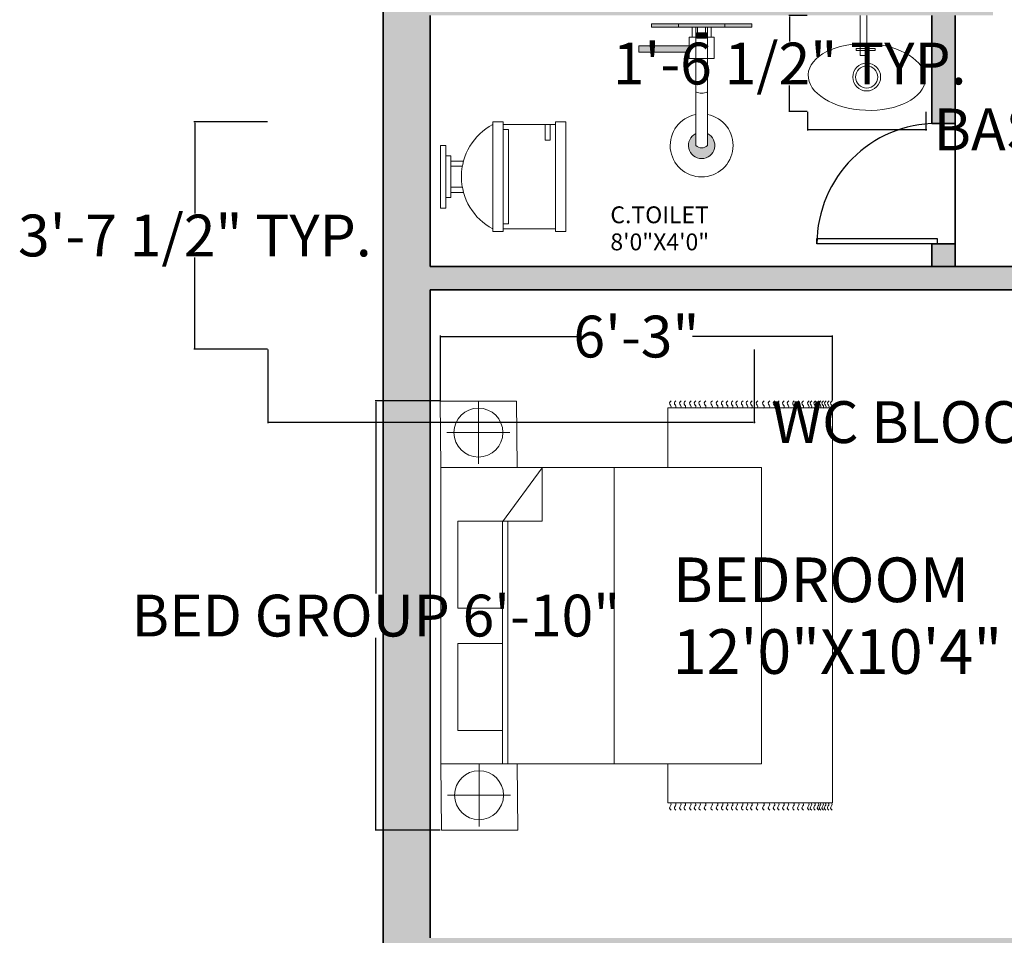
# Model space of a CAD drawing. Units: inches. Extents: x -4737294 to -4736756, y 1716389 to 1717040.
# Tile 17 of 25: x -4737285 to -4737096, y 1716669 to 1716844. Entities that reach past the tile are written whole.
import ezdxf

# ---------------------------------------------------------------- set-up
doc = ezdxf.new("R2010")
doc.units = ezdxf.units.IN
doc.header["$MEASUREMENT"] = 0
for name, color, linetype, lineweight in [('A-ANNO-DIMS', 2, 'Continuous', 18), ('A-AREA-IDEN', 250, 'Continuous', 18), ('A-WALL-PATT', 244, 'Continuous', 13), ('doors', 252, 'Continuous', 25), ('furniture', 250, 'Continuous', 18), ('PLUMBING FIXTURES', 252, 'Continuous', 18), ('walls', 252, 'Continuous', 35)]:
    doc.layers.add(name, color=color, linetype=linetype, lineweight=lineweight)
doc.styles.get("Standard").update_dxf_attribs({"font": 'arial.ttf'})
doc.dimstyles.get("Standard").update_dxf_attribs({"dimtxt": 8, "dimasz": 0.18, "dimexe": 0.18, "dimexo": 0.0625, "dimgap": 0.09, "dimtad": 0, "dimtih": 1, "dimtoh": 1, "dimzin": 0, "dimdsep": 46, "dimlunit": 3, "dimtxsty": 'Standard', "dimcen": 0.09, "dimadec": 0, "dimazin": 0, "dimtfac": 1, "dimtofl": 0, "dimtmove": 0, "dimatfit": 3, "dimfxl": 1, "dimtolj": 1, "dimtzin": 0, "dimarcsym": 0})

# ---------------------------------------------------------------- blocks, each defined once
blk = doc.blocks.new('O.H SHOWER-PL')
at = {"layer": 'PLUMBING FIXTURES'}
for points in [[(-1.838, 0), (-1.838, -0.25), (1.838, -0.25), (1.838, 0)], [(0.461, -8.724), (0.461, -9.667, -0.422337), (-0.461, -9.667), (-0.461, -8.724, 4.325472)]]:
    blk.add_hatch(color=256, dxfattribs=at).paths.add_polyline_path(points)
for p, q in [((-1.838, 0), (-1.838, -0.25)), ((1.838, 0), (-1.838, 0)), ((1.838, 0), (1.838, -0.25)), ((1.838, -0.25), (-1.838, -0.25)), ((-0.461, -0.25), (-0.461, -9.667)), ((0.461, -0.25), (0.461, -9.667))]:
    blk.add_line(p, q, dxfattribs=at)
for centre, radius, start, end in [((0, -4.479), 1.033, 243.52996, 296.47004), ((0, -9.667), 2.501, 100.61004, 79.38997), ((0, -9.667), 1.049, 116.03487, 63.96515), ((0, -9.219), 0.643, 224.20776, 315.79224)]:
    blk.add_arc(centre, radius, start, end, dxfattribs=at)
blk = doc.blocks.new('DIVERTER-PL')
at = {"layer": 'PLUMBING FIXTURES'}
for points in [[(4, 0), (-4, 0), (-4, -0.25), (4, -0.25)], [(0.375, -1.144), (0.375, -0.704), (-0.375, -0.704), (-0.375, -1.144)], [(1, -1.751, 0.30818), (1, -2.251), (5, -2.251), (5, -1.751)]]:
    blk.add_hatch(color=256, dxfattribs=at).paths.add_polyline_path(points)
for p, q in [((-4, 0), (-4, -0.25)), ((-4, 0), (4, 0)), ((4, 0), (4, -0.25)), ((-4, -0.25), (4, -0.25)), ((-4, -0.25), (4, -0.25)), ((-0.75, -0.25), (-0.75, -1.05)), ((-0.375, -0.704), (0.375, -0.704)), ((-0.375, -0.704), (-0.375, -1.144)), ((-0.318, -0.704), (-0.318, -0.25)), ((0.318, -0.704), (0.318, -0.25)), ((0.375, -0.704), (0.375, -1.144)), ((0.75, -0.25), (0.75, -1.05)), ((-1, -1.05), (-0.375, -1.05)), ((-1, -1.05), (-1, -2.75)), ((-0.375, -1.144), (0.375, -1.144)), ((0.375, -1.05), (1, -1.05)), ((1, -1.05), (1, -1.751)), ((1, -2.251), (1, -2.75)), ((-1, -2.75), (1, -2.75))]:
    blk.add_line(p, q, dxfattribs=at)
at = {"layer": 'PLUMBING FIXTURES', "ltscale": 12}
for p, q in [((1, -1.751), (5, -1.751)), ((1, -2.251), (5, -2.251)), ((5, -2.251), (5, -1.751))]:
    blk.add_line(p, q, dxfattribs=at)
at = {"layer": 'PLUMBING FIXTURES'}
blk.add_arc((1.367, -2.001), 0.444, 145.74346, 214.25654, dxfattribs=at)
blk = doc.blocks.new('A$C7F153053')
at = {"layer": 'PLUMBING FIXTURES', "xscale": -1, "rotation": 270}
for name in ['DIVERTER-PL', 'O.H SHOWER-PL']:
    blk.add_blockref(name, (12.166, 4), dxfattribs=at)
blk = doc.blocks.new('CARPET')
at = {"layer": 'furniture'}
for p, q in [((-51.53, -98.11), (-51.53, -55.12)), ((-51.53, -55.12), (-41.27, -55.12)), ((36, -55.12), (51.55, -55.12)), ((51.55, -55.12), (51.55, -98.11)), ((51.55, -98.11), (-51.53, -98.11))]:
    blk.add_line(p, q, dxfattribs=at)
for points, knots in [([(-53.37, -55.99), (-53.22, -55.8), (-52.9, -55.41), (-52.34, -55.8), (-51.89, -56.08), (-51.65, -55.91), (-51.53, -55.83)], [0, 0, 0, 0, 0.653278, 1.290138, 1.740457, 2.114451, 2.114451, 2.114451, 2.114451]), ([(53.37, -55.99), (53.22, -55.8), (52.9, -55.41), (52.34, -55.8), (51.89, -56.08), (51.65, -55.91), (51.53, -55.83)], [0, 0, 0, 0, 0.653278, 1.290138, 1.740457, 2.114451, 2.114451, 2.114451, 2.114451]), ([(-53.37, -57.26), (-53.22, -57.07), (-52.9, -56.67), (-52.34, -57.07), (-51.89, -57.35), (-51.65, -57.17), (-51.53, -57.1)], [0, 0, 0, 0, 0.653278, 1.290138, 1.740457, 2.114451, 2.114451, 2.114451, 2.114451]), ([(-53.37, -58.59), (-53.22, -58.4), (-52.9, -58.01), (-52.34, -58.4), (-51.89, -58.68), (-51.65, -58.5), (-51.53, -58.43)], [0, 0, 0, 0, 0.653278, 1.290138, 1.740457, 2.114451, 2.114451, 2.114451, 2.114451]), ([(53.37, -57.26), (53.22, -57.07), (52.9, -56.67), (52.34, -57.07), (51.89, -57.35), (51.65, -57.17), (51.53, -57.1)], [0, 0, 0, 0, 0.653278, 1.290138, 1.740457, 2.114451, 2.114451, 2.114451, 2.114451]), ([(53.37, -58.59), (53.22, -58.4), (52.9, -58.01), (52.34, -58.4), (51.89, -58.68), (51.65, -58.5), (51.53, -58.43)], [0, 0, 0, 0, 0.653278, 1.290138, 1.740457, 2.114451, 2.114451, 2.114451, 2.114451]), ([(-53.37, -59.78), (-53.22, -59.58), (-52.9, -59.19), (-52.34, -59.58), (-51.89, -59.86), (-51.65, -59.69), (-51.53, -59.61)], [0, 0, 0, 0, 0.653278, 1.290138, 1.740457, 2.114451, 2.114451, 2.114451, 2.114451]), ([(-53.37, -61.22), (-53.22, -61.02), (-52.9, -60.63), (-52.34, -61.02), (-51.89, -61.3), (-51.65, -61.13), (-51.53, -61.05)], [0, 0, 0, 0, 0.653278, 1.290138, 1.740457, 2.114451, 2.114451, 2.114451, 2.114451]), ([(53.37, -59.78), (53.22, -59.58), (52.9, -59.19), (52.34, -59.58), (51.89, -59.86), (51.65, -59.69), (51.53, -59.61)], [0, 0, 0, 0, 0.653278, 1.290138, 1.740457, 2.114451, 2.114451, 2.114451, 2.114451]), ([(53.37, -61.22), (53.22, -61.02), (52.9, -60.63), (52.34, -61.02), (51.89, -61.3), (51.65, -61.13), (51.53, -61.05)], [0, 0, 0, 0, 0.653278, 1.290138, 1.740457, 2.114451, 2.114451, 2.114451, 2.114451]), ([(-53.37, -62.44), (-53.22, -62.25), (-52.9, -61.86), (-52.34, -62.25), (-51.89, -62.53), (-51.65, -62.36), (-51.53, -62.28)], [0, 0, 0, 0, 0.653278, 1.290138, 1.740457, 2.114451, 2.114451, 2.114451, 2.114451]), ([(-53.37, -63.63), (-53.22, -63.43), (-52.9, -63.04), (-52.34, -63.43), (-51.89, -63.72), (-51.65, -63.54), (-51.53, -63.46)], [0, 0, 0, 0, 0.653278, 1.290138, 1.740457, 2.114451, 2.114451, 2.114451, 2.114451]), ([(53.37, -62.44), (53.22, -62.25), (52.9, -61.86), (52.34, -62.25), (51.89, -62.53), (51.65, -62.36), (51.53, -62.28)], [0, 0, 0, 0, 0.653278, 1.290138, 1.740457, 2.114451, 2.114451, 2.114451, 2.114451]), ([(53.37, -63.63), (53.22, -63.43), (52.9, -63.04), (52.34, -63.43), (51.89, -63.72), (51.65, -63.54), (51.53, -63.46)], [0, 0, 0, 0, 0.653278, 1.290138, 1.740457, 2.114451, 2.114451, 2.114451, 2.114451]), ([(-53.37, -65.07), (-53.22, -64.87), (-52.9, -64.48), (-52.34, -64.87), (-51.89, -65.15), (-51.65, -64.98), (-51.53, -64.9)], [0, 0, 0, 0, 0.653278, 1.290138, 1.740457, 2.114451, 2.114451, 2.114451, 2.114451]), ([(-53.37, -66.76), (-53.22, -66.56), (-52.9, -66.17), (-52.34, -66.56), (-51.89, -66.84), (-51.65, -66.67), (-51.53, -66.59)], [0, 0, 0, 0, 0.653278, 1.290138, 1.740457, 2.114451, 2.114451, 2.114451, 2.114451]), ([(53.37, -65.07), (53.22, -64.87), (52.9, -64.48), (52.34, -64.87), (51.89, -65.15), (51.65, -64.98), (51.53, -64.9)], [0, 0, 0, 0, 0.653278, 1.290138, 1.740457, 2.114451, 2.114451, 2.114451, 2.114451]), ([(53.37, -66.76), (53.22, -66.56), (52.9, -66.17), (52.34, -66.56), (51.89, -66.84), (51.65, -66.67), (51.53, -66.59)], [0, 0, 0, 0, 0.653278, 1.290138, 1.740457, 2.114451, 2.114451, 2.114451, 2.114451]), ([(-53.37, -68.2), (-53.22, -68), (-52.9, -67.61), (-52.34, -68), (-51.89, -68.28), (-51.65, -68.11), (-51.53, -68.03)], [0, 0, 0, 0, 0.653278, 1.290138, 1.740457, 2.114451, 2.114451, 2.114451, 2.114451]), ([(-53.37, -69.53), (-53.22, -69.33), (-52.9, -68.94), (-52.34, -69.33), (-51.89, -69.61), (-51.65, -69.44), (-51.53, -69.36)], [0, 0, 0, 0, 0.653278, 1.290138, 1.740457, 2.114451, 2.114451, 2.114451, 2.114451]), ([(53.37, -68.2), (53.22, -68), (52.9, -67.61), (52.34, -68), (51.89, -68.28), (51.65, -68.11), (51.53, -68.03)], [0, 0, 0, 0, 0.653278, 1.290138, 1.740457, 2.114451, 2.114451, 2.114451, 2.114451]), ([(53.37, -69.53), (53.22, -69.33), (52.9, -68.94), (52.34, -69.33), (51.89, -69.61), (51.65, -69.44), (51.53, -69.36)], [0, 0, 0, 0, 0.653278, 1.290138, 1.740457, 2.114451, 2.114451, 2.114451, 2.114451]), ([(-53.37, -70.79), (-53.22, -70.6), (-52.9, -70.21), (-52.34, -70.6), (-51.89, -70.88), (-51.65, -70.7), (-51.53, -70.63)], [0, 0, 0, 0, 0.653278, 1.290138, 1.740457, 2.114451, 2.114451, 2.114451, 2.114451]), ([(-53.37, -72.12), (-53.22, -71.93), (-52.9, -71.54), (-52.34, -71.93), (-51.89, -72.21), (-51.65, -72.04), (-51.53, -71.96)], [0, 0, 0, 0, 0.653278, 1.290138, 1.740457, 2.114451, 2.114451, 2.114451, 2.114451]), ([(53.37, -70.79), (53.22, -70.6), (52.9, -70.21), (52.34, -70.6), (51.89, -70.88), (51.65, -70.7), (51.53, -70.63)], [0, 0, 0, 0, 0.653278, 1.290138, 1.740457, 2.114451, 2.114451, 2.114451, 2.114451]), ([(53.37, -72.12), (53.22, -71.93), (52.9, -71.54), (52.34, -71.93), (51.89, -72.21), (51.65, -72.04), (51.53, -71.96)], [0, 0, 0, 0, 0.653278, 1.290138, 1.740457, 2.114451, 2.114451, 2.114451, 2.114451]), ([(-53.37, -73.31), (-53.22, -73.11), (-52.9, -72.72), (-52.34, -73.11), (-51.89, -73.4), (-51.65, -73.22), (-51.53, -73.14)], [0, 0, 0, 0, 0.653278, 1.290138, 1.740457, 2.114451, 2.114451, 2.114451, 2.114451]), ([(-53.37, -74.75), (-53.22, -74.55), (-52.9, -74.16), (-52.34, -74.55), (-51.89, -74.83), (-51.65, -74.66), (-51.53, -74.58)], [0, 0, 0, 0, 0.653278, 1.290138, 1.740457, 2.114451, 2.114451, 2.114451, 2.114451]), ([(53.37, -73.31), (53.22, -73.11), (52.9, -72.72), (52.34, -73.11), (51.89, -73.4), (51.65, -73.22), (51.53, -73.14)], [0, 0, 0, 0, 0.653278, 1.290138, 1.740457, 2.114451, 2.114451, 2.114451, 2.114451]), ([(53.37, -74.75), (53.22, -74.55), (52.9, -74.16), (52.34, -74.55), (51.89, -74.83), (51.65, -74.66), (51.53, -74.58)], [0, 0, 0, 0, 0.653278, 1.290138, 1.740457, 2.114451, 2.114451, 2.114451, 2.114451]), ([(-53.37, -75.98), (-53.22, -75.78), (-52.9, -75.39), (-52.34, -75.78), (-51.89, -76.06), (-51.65, -75.89), (-51.53, -75.81)], [0, 0, 0, 0, 0.653278, 1.290138, 1.740457, 2.114451, 2.114451, 2.114451, 2.114451]), ([(-53.37, -77.16), (-53.22, -76.96), (-52.9, -76.57), (-52.34, -76.96), (-51.89, -77.25), (-51.65, -77.07), (-51.53, -76.99)], [0, 0, 0, 0, 0.653278, 1.290138, 1.740457, 2.114451, 2.114451, 2.114451, 2.114451]), ([(53.37, -75.98), (53.22, -75.78), (52.9, -75.39), (52.34, -75.78), (51.89, -76.06), (51.65, -75.89), (51.53, -75.81)], [0, 0, 0, 0, 0.653278, 1.290138, 1.740457, 2.114451, 2.114451, 2.114451, 2.114451]), ([(53.37, -77.16), (53.22, -76.96), (52.9, -76.57), (52.34, -76.96), (51.89, -77.25), (51.65, -77.07), (51.53, -76.99)], [0, 0, 0, 0, 0.653278, 1.290138, 1.740457, 2.114451, 2.114451, 2.114451, 2.114451]), ([(-53.37, -78.6), (-53.22, -78.4), (-52.9, -78.01), (-52.34, -78.4), (-51.89, -78.68), (-51.65, -78.51), (-51.53, -78.43)], [0, 0, 0, 0, 0.653278, 1.290138, 1.740457, 2.114451, 2.114451, 2.114451, 2.114451]), ([(53.37, -78.6), (53.22, -78.4), (52.9, -78.01), (52.34, -78.4), (51.89, -78.68), (51.65, -78.51), (51.53, -78.43)], [0, 0, 0, 0, 0.653278, 1.290138, 1.740457, 2.114451, 2.114451, 2.114451, 2.114451]), ([(-53.37, -80.29), (-53.22, -80.09), (-52.9, -79.7), (-52.34, -80.09), (-51.89, -80.37), (-51.65, -80.2), (-51.53, -80.12)], [0, 0, 0, 0, 0.653278, 1.290138, 1.740457, 2.114451, 2.114451, 2.114451, 2.114451]), ([(-53.37, -81.73), (-53.22, -81.53), (-52.9, -81.14), (-52.34, -81.53), (-51.89, -81.81), (-51.65, -81.64), (-51.53, -81.56)], [0, 0, 0, 0, 0.653278, 1.290138, 1.740457, 2.114451, 2.114451, 2.114451, 2.114451]), ([(53.37, -80.29), (53.22, -80.09), (52.9, -79.7), (52.34, -80.09), (51.89, -80.37), (51.65, -80.2), (51.53, -80.12)], [0, 0, 0, 0, 0.653278, 1.290138, 1.740457, 2.114451, 2.114451, 2.114451, 2.114451]), ([(53.37, -81.73), (53.22, -81.53), (52.9, -81.14), (52.34, -81.53), (51.89, -81.81), (51.65, -81.64), (51.53, -81.56)], [0, 0, 0, 0, 0.653278, 1.290138, 1.740457, 2.114451, 2.114451, 2.114451, 2.114451]), ([(-53.37, -83.06), (-53.22, -82.86), (-52.9, -82.47), (-52.34, -82.86), (-51.89, -83.14), (-51.65, -82.97), (-51.53, -82.89)], [0, 0, 0, 0, 0.653278, 1.290138, 1.740457, 2.114451, 2.114451, 2.114451, 2.114451]), ([(-53.37, -84.18), (-53.22, -83.99), (-52.9, -83.6), (-52.34, -83.99), (-51.89, -84.27), (-51.65, -84.09), (-51.53, -84.02)], [0, 0, 0, 0, 0.653278, 1.290138, 1.740457, 2.114451, 2.114451, 2.114451, 2.114451]), ([(53.37, -83.06), (53.22, -82.86), (52.9, -82.47), (52.34, -82.86), (51.89, -83.14), (51.65, -82.97), (51.53, -82.89)], [0, 0, 0, 0, 0.653278, 1.290138, 1.740457, 2.114451, 2.114451, 2.114451, 2.114451]), ([(53.37, -84.18), (53.22, -83.99), (52.9, -83.6), (52.34, -83.99), (51.89, -84.27), (51.65, -84.09), (51.53, -84.02)], [0, 0, 0, 0, 0.653278, 1.290138, 1.740457, 2.114451, 2.114451, 2.114451, 2.114451]), ([(-53.37, -85.51), (-53.22, -85.32), (-52.9, -84.93), (-52.34, -85.32), (-51.89, -85.6), (-51.65, -85.42), (-51.53, -85.35)], [0, 0, 0, 0, 0.653278, 1.290138, 1.740457, 2.114451, 2.114451, 2.114451, 2.114451]), ([(-53.37, -86.7), (-53.22, -86.5), (-52.9, -86.11), (-52.34, -86.5), (-51.89, -86.78), (-51.65, -86.61), (-51.53, -86.53)], [0, 0, 0, 0, 0.653278, 1.290138, 1.740457, 2.114451, 2.114451, 2.114451, 2.114451]), ([(53.37, -85.51), (53.22, -85.32), (52.9, -84.93), (52.34, -85.32), (51.89, -85.6), (51.65, -85.42), (51.53, -85.35)], [0, 0, 0, 0, 0.653278, 1.290138, 1.740457, 2.114451, 2.114451, 2.114451, 2.114451]), ([(53.37, -86.7), (53.22, -86.5), (52.9, -86.11), (52.34, -86.5), (51.89, -86.78), (51.65, -86.61), (51.53, -86.53)], [0, 0, 0, 0, 0.653278, 1.290138, 1.740457, 2.114451, 2.114451, 2.114451, 2.114451]), ([(-53.37, -88.14), (-53.22, -87.94), (-52.9, -87.55), (-52.34, -87.94), (-51.89, -88.22), (-51.65, -88.05), (-51.53, -87.97)], [0, 0, 0, 0, 0.653278, 1.290138, 1.740457, 2.114451, 2.114451, 2.114451, 2.114451]), ([(-53.37, -89.36), (-53.22, -89.17), (-52.9, -88.78), (-52.34, -89.17), (-51.89, -89.45), (-51.65, -89.28), (-51.53, -89.2)], [0, 0, 0, 0, 0.653278, 1.290138, 1.740457, 2.114451, 2.114451, 2.114451, 2.114451]), ([(53.37, -88.14), (53.22, -87.94), (52.9, -87.55), (52.34, -87.94), (51.89, -88.22), (51.65, -88.05), (51.53, -87.97)], [0, 0, 0, 0, 0.653278, 1.290138, 1.740457, 2.114451, 2.114451, 2.114451, 2.114451]), ([(53.37, -89.36), (53.22, -89.17), (52.9, -88.78), (52.34, -89.17), (51.89, -89.45), (51.65, -89.28), (51.53, -89.2)], [0, 0, 0, 0, 0.653278, 1.290138, 1.740457, 2.114451, 2.114451, 2.114451, 2.114451]), ([(-53.37, -90.55), (-53.22, -90.35), (-52.9, -89.96), (-52.34, -90.35), (-51.89, -90.64), (-51.65, -90.46), (-51.53, -90.38)], [0, 0, 0, 0, 0.653278, 1.290138, 1.740457, 2.114451, 2.114451, 2.114451, 2.114451]), ([(-53.37, -91.99), (-53.22, -91.79), (-52.9, -91.4), (-52.34, -91.79), (-51.89, -92.07), (-51.65, -91.9), (-51.53, -91.82)], [0, 0, 0, 0, 0.653278, 1.290138, 1.740457, 2.114451, 2.114451, 2.114451, 2.114451]), ([(-53.37, -92.69), (-53.22, -92.48), (-52.9, -92.08), (-52.35, -92.49), (-51.89, -92.77), (-51.65, -92.6), (-51.53, -92.52)], [0, 0, 0, 0, 0.663904, 1.307406, 1.757725, 2.131719, 2.131719, 2.131719, 2.131719]), ([(53.37, -90.55), (53.22, -90.35), (52.9, -89.96), (52.34, -90.35), (51.9, -90.63), (51.66, -90.47), (51.55, -90.4)], [0, 0, 0, 0, 0.653278, 1.290138, 1.740457, 2.0926, 2.0926, 2.0926, 2.0926]), ([(53.37, -91.99), (53.22, -91.79), (52.9, -91.4), (52.34, -91.79), (51.9, -92.07), (51.66, -91.91), (51.55, -91.83)], [0, 0, 0, 0, 0.653278, 1.290138, 1.740457, 2.0926, 2.0926, 2.0926, 2.0926]), ([(53.37, -92.69), (53.22, -92.49), (52.9, -92.09), (52.34, -92.49), (51.9, -92.77), (51.66, -92.61), (51.55, -92.53)], [0, 0, 0, 0, 0.656792, 1.295826, 1.746145, 2.098292, 2.098292, 2.098292, 2.098292]), ([(-53.37, -93.61), (-53.22, -93.42), (-52.9, -93.03), (-52.34, -93.42), (-51.89, -93.7), (-51.65, -93.52), (-51.53, -93.45)], [0, 0, 0, 0, 0.653278, 1.290138, 1.740457, 2.114451, 2.114451, 2.114451, 2.114451]), ([(-53.37, -94.55), (-53.22, -94.35), (-52.9, -93.96), (-52.34, -94.35), (-51.89, -94.63), (-51.65, -94.46), (-51.53, -94.38)], [0, 0, 0, 0, 0.653278, 1.290138, 1.740457, 2.114451, 2.114451, 2.114451, 2.114451]), ([(-53.37, -95.05), (-53.22, -94.85), (-52.9, -94.46), (-52.34, -94.85), (-51.89, -95.14), (-51.65, -94.96), (-51.53, -94.88)], [0, 0, 0, 0, 0.653278, 1.290138, 1.740457, 2.114451, 2.114451, 2.114451, 2.114451]), ([(53.37, -93.66), (53.22, -93.46), (52.9, -93.07), (52.34, -93.46), (51.9, -93.74), (51.66, -93.58), (51.55, -93.5)], [0, 0, 0, 0, 0.653278, 1.290138, 1.740457, 2.0926, 2.0926, 2.0926, 2.0926]), ([(53.37, -94.59), (53.22, -94.4), (52.9, -94.01), (52.34, -94.4), (51.9, -94.68), (51.66, -94.51), (51.55, -94.44)], [0, 0, 0, 0, 0.653278, 1.290138, 1.740457, 2.0926, 2.0926, 2.0926, 2.0926]), ([(53.37, -95.1), (53.22, -94.9), (52.9, -94.51), (52.34, -94.9), (51.9, -95.18), (51.66, -95.02), (51.55, -94.94)], [0, 0, 0, 0, 0.653278, 1.290138, 1.740457, 2.0926, 2.0926, 2.0926, 2.0926]), ([(-53.37, -95.73), (-53.22, -95.54), (-52.9, -95.15), (-52.34, -95.54), (-51.89, -95.82), (-51.65, -95.65), (-51.53, -95.57)], [0, 0, 0, 0, 0.653278, 1.290138, 1.740457, 2.114451, 2.114451, 2.114451, 2.114451]), ([(-53.37, -96.38), (-53.22, -96.18), (-52.9, -95.79), (-52.34, -96.18), (-51.89, -96.47), (-51.65, -96.29), (-51.53, -96.21)], [0, 0, 0, 0, 0.653278, 1.290138, 1.740457, 2.114451, 2.114451, 2.114451, 2.114451]), ([(-53.37, -97.17), (-53.22, -96.98), (-52.9, -96.59), (-52.34, -96.98), (-51.89, -97.26), (-51.65, -97.08), (-51.53, -97.01)], [0, 0, 0, 0, 0.653278, 1.290138, 1.740457, 2.114451, 2.114451, 2.114451, 2.114451]), ([(-53.37, -97.99), (-53.22, -97.79), (-52.9, -97.4), (-52.34, -97.79), (-51.89, -98.08), (-51.65, -97.9), (-51.53, -97.82)], [0, 0, 0, 0, 0.653278, 1.290138, 1.740457, 2.114451, 2.114451, 2.114451, 2.114451]), ([(53.37, -95.78), (53.22, -95.58), (52.9, -95.19), (52.34, -95.58), (51.89, -95.86), (51.65, -95.69), (51.53, -95.61)], [0, 0, 0, 0, 0.653278, 1.290138, 1.740457, 2.114451, 2.114451, 2.114451, 2.114451]), ([(53.37, -96.43), (53.22, -96.23), (52.9, -95.84), (52.34, -96.23), (51.89, -96.51), (51.65, -96.34), (51.53, -96.26)], [0, 0, 0, 0, 0.653278, 1.290138, 1.740457, 2.114451, 2.114451, 2.114451, 2.114451]), ([(53.37, -97.22), (53.22, -97.02), (52.9, -96.63), (52.34, -97.02), (51.89, -97.3), (51.65, -97.13), (51.53, -97.05)], [0, 0, 0, 0, 0.653278, 1.290138, 1.740457, 2.114451, 2.114451, 2.114451, 2.114451]), ([(53.37, -97.99), (53.22, -97.79), (52.9, -97.4), (52.34, -97.79), (51.89, -98.08), (51.65, -97.9), (51.53, -97.82)], [0, 0, 0, 0, 0.653278, 1.290138, 1.740457, 2.114451, 2.114451, 2.114451, 2.114451])]:
    blk.add_open_spline(points, degree=3, knots=knots, dxfattribs=at)
blk = doc.blocks.new('A$C58D270C6')
at = {"layer": 'furniture'}
for p, q in [((9.09, 124.13), (9.09, 108.87)), ((1.46, 116.5), (16.73, 116.5)), ((14.97, 94.84), (24.62, 107.92)), ((24.62, 94.93), (24.62, 107.92)), ((42.08, 108), (42.08, 36)), ((14.97, 94.93), (24.62, 94.93)), ((14.97, 94.84), (14.97, 36)), ((16.22, 94.93), (16.22, 36)), ((9.25, 36), (9.25, 20.74)), ((1.62, 28.37), (16.88, 28.37))]:
    blk.add_line(p, q, dxfattribs=at)
for points in [[(18.5, 108), (18.34, 124.13), (-0.16, 124.13), (0, 108)], [(0, 108), (77.91, 108), (77.91, 36), (0, 36)], [(4.09, 94.93), (14.97, 94.93), (14.97, 73.83), (4.09, 73.83)], [(4.09, 65.23), (14.97, 65.23), (14.97, 44.13), (4.09, 44.13)], [(18.65, 19.87), (18.5, 36), (0, 36), (0.16, 19.87)]]:
    blk.add_lwpolyline(points, close=True, dxfattribs=at)
for centre in [(9.09, 116.5), (9.25, 28.37)]:
    blk.add_circle(centre, 5.95, dxfattribs=at)
at = {"layer": 'furniture', "xscale": 0.9312884925094044, "yscale": 0.9312884925094044, "zscale": 0.9312884925094044, "rotation": 90}
blk.add_blockref('CARPET', (3.79, 74.47), dxfattribs=at)
blk = doc.blocks.new('Toilet - Imperial')
for p, q in [((-10, 22), (-10, 12)), ((-10, 21), (-7, 21)), ((-7, 21), (-7, 20)), ((10, 12), (10, 22)), ((-7, 20), (-10, 20)), ((10.5, 12), (-10.5, 12)), ((-10.5, 10), (-10.5, 12)), ((9, 13), (-9, 13)), ((-9, 13), (-9, 12)), ((9, 12), (9, 13)), ((10.5, 12), (10.5, 10)), ((10.5, 10), (-10.5, 10)), ((-3, 4.4065), (-3, 2)), ((-2, 2), (-2, 4.1658)), ((2, 4.1658), (2, 2)), ((3, 2), (3, 4.4065)), ((4, 2), (-4, 2)), ((-4, 2), (-4, 1)), ((4, 1), (4, 2))]:
    blk.add_line(p, q)
for points in [[(10.5, 22), (10.5, 24), (-10.5, 24), (-10.5, 22)], [(6, 0), (6, 1), (-6, 1), (-6, 0)]]:
    blk.add_lwpolyline(points, close=True)
blk.add_arc((0, 15.3333), 11.3333, 208.0725, 331.9275)
blk = doc.blocks.new('*U20')
for p, q in [((0, 0), (0, -6)), ((40, 0), (40, -6))]:
    blk.add_line(p, q)
blk.add_lwpolyline([(0, 0), (0, 40), (1.75, 40), (1.75, 0)], close=True)
blk.add_arc((0, 0), 40, 0, 90)
blk = doc.blocks.new('LAVATORY-OVAL-WITH-TAP')
for p, q in [((6.3, 12.81), (6.3, 9.15)), ((6.71, 12.81), (6.3, 12.81)), ((6.71, 9.15), (6.71, 12.81)), ((0, 11.19), (7.64, 11.19)), ((7.64, 9.95), (0, 9.95)), ((7.64, 11.19), (7.64, 9.95)), ((6.3, 9.15), (6.71, 9.15))]:
    blk.add_line(p, q)
for radius in [2.67, 2.13, 2.13, 2.13]:
    blk.add_circle((11.77, 11.19), radius)
blk.add_ellipse((11.77, 11.19), major_axis=(-0.46, -11.19), ratio=0.56899)
blk = doc.blocks.new('*D33')
at = {"layer": 'A-ANNO-DIMS', "color": 0, "lineweight": -2, "transparency": 16777216}
for p, q in [((-4737204.24, 1716770.81), (-4737216.68, 1716770.81)), ((-4737216.5, 1716770.63), (-4737216.5, 1716733.97)), ((-4737216.5, 1716688.86), (-4737216.5, 1716725.51)), ((-4737204.24, 1716688.68), (-4737216.68, 1716688.68))]:
    blk.add_line(p, q, dxfattribs=at)
at = {"layer": 'A-ANNO-DIMS', "color": 0, "transparency": 16777216}
for points in [[(-4737216.53, 1716770.63), (-4737216.47, 1716770.63), (-4737216.5, 1716770.81)], [(-4737216.53, 1716688.86), (-4737216.47, 1716688.86), (-4737216.5, 1716688.68)]]:
    blk.add_solid(points, dxfattribs=at)
at = {"layer": 'Defpoints', "color": 0, "transparency": 16777216}
for p in [(-4737216.5, 1716770.81), (-4737204.18, 1716770.81), (-4737204.18, 1716688.68)]:
    blk.add_point(p, dxfattribs=at)
at = {"layer": 'A-ANNO-DIMS', "color": 0, "transparency": 16777216, "insert": (-4737216.5, 1716729.74), "char_height": 8, "attachment_point": 5}
blk.add_mtext('\\A1;BED GROUP 6\'-10"', dxfattribs=at)
blk = doc.blocks.new('*D34')
at = {"layer": 'A-ANNO-DIMS', "color": 0, "lineweight": -2, "transparency": 16777216}
for p, q in [((-4737204.18, 1716770.87), (-4737204.18, 1716783.31)), ((-4737204, 1716783.13), (-4737177.41, 1716783.13)), ((-4737129.32, 1716783.13), (-4737155.92, 1716783.13)), ((-4737129.14, 1716770.87), (-4737129.14, 1716783.31))]:
    blk.add_line(p, q, dxfattribs=at)
at = {"layer": 'A-ANNO-DIMS', "color": 0, "transparency": 16777216}
for points in [[(-4737204, 1716783.16), (-4737204, 1716783.1), (-4737204.18, 1716783.13)], [(-4737129.32, 1716783.16), (-4737129.32, 1716783.1), (-4737129.14, 1716783.13)]]:
    blk.add_solid(points, dxfattribs=at)
at = {"layer": 'Defpoints', "color": 0, "transparency": 16777216}
for p in [(-4737129.14, 1716783.13), (-4737204.18, 1716770.81), (-4737129.14, 1716770.81)]:
    blk.add_point(p, dxfattribs=at)
at = {"layer": 'A-ANNO-DIMS', "color": 0, "transparency": 16777216, "insert": (-4737166.66, 1716783.13), "char_height": 8, "attachment_point": 5}
blk.add_mtext('\\A1;6\'-3"', dxfattribs=at)
blk = doc.blocks.new('*D37')
at = {"layer": 'A-ANNO-DIMS', "color": 0, "lineweight": -2, "transparency": 16777216}
for p, q in [((-4737237.19, 1716780.66), (-4737237.19, 1716766.58)), ((-4737144.14, 1716780.66), (-4737144.14, 1716766.58)), ((-4737237.01, 1716766.76), (-4737144.32, 1716766.76)), ((-4737144.14, 1716766.76), (-4737143.96, 1716766.76))]:
    blk.add_line(p, q, dxfattribs=at)
at = {"layer": 'A-ANNO-DIMS', "color": 0, "transparency": 16777216}
for points in [[(-4737237.01, 1716766.79), (-4737237.01, 1716766.73), (-4737237.19, 1716766.76)], [(-4737144.32, 1716766.79), (-4737144.32, 1716766.73), (-4737144.14, 1716766.76)]]:
    blk.add_solid(points, dxfattribs=at)
at = {"layer": 'Defpoints', "color": 0, "transparency": 16777216}
for p in [(-4737237.19, 1716780.72), (-4737144.14, 1716780.72), (-4737144.14, 1716766.76)]:
    blk.add_point(p, dxfattribs=at)
at = {"layer": 'A-ANNO-DIMS', "color": 0, "transparency": 16777216, "insert": (-4737087.97, 1716766.76), "char_height": 8, "attachment_point": 5}
blk.add_mtext('\\A1;WC BLOCK 7\'-9" TYP.', dxfattribs=at)
blk = doc.blocks.new('*D38')
at = {"layer": 'A-ANNO-DIMS', "color": 0, "lineweight": -2, "transparency": 16777216}
for p, q in [((-4737237.25, 1716824.22), (-4737251.33, 1716824.22)), ((-4737251.15, 1716824.04), (-4737251.15, 1716806.7)), ((-4737251.15, 1716780.9), (-4737251.15, 1716798.24)), ((-4737237.25, 1716780.72), (-4737251.33, 1716780.72))]:
    blk.add_line(p, q, dxfattribs=at)
at = {"layer": 'A-ANNO-DIMS', "color": 0, "transparency": 16777216}
for points in [[(-4737251.18, 1716824.04), (-4737251.12, 1716824.04), (-4737251.15, 1716824.22)], [(-4737251.18, 1716780.9), (-4737251.12, 1716780.9), (-4737251.15, 1716780.72)]]:
    blk.add_solid(points, dxfattribs=at)
at = {"layer": 'Defpoints', "color": 0, "transparency": 16777216}
for p in [(-4737237.19, 1716824.22), (-4737251.15, 1716780.72), (-4737237.19, 1716780.72)]:
    blk.add_point(p, dxfattribs=at)
at = {"layer": 'A-ANNO-DIMS', "color": 0, "transparency": 16777216, "insert": (-4737251.15, 1716802.47), "char_height": 8, "attachment_point": 5}
blk.add_mtext('\\A1;3\'-7 1/2" TYP.', dxfattribs=at)
blk = doc.blocks.new('*D41')
at = {"layer": 'A-ANNO-DIMS', "color": 0, "lineweight": -2, "transparency": 16777216}
for p, q in [((-4737133.94, 1716826.11), (-4737133.94, 1716822.59)), ((-4737111.26, 1716826.11), (-4737111.26, 1716822.59)), ((-4737133.76, 1716822.77), (-4737111.44, 1716822.77)), ((-4737111.26, 1716822.77), (-4737111.08, 1716822.77))]:
    blk.add_line(p, q, dxfattribs=at)
at = {"layer": 'A-ANNO-DIMS', "color": 0, "transparency": 16777216}
for points in [[(-4737133.76, 1716822.8), (-4737133.76, 1716822.74), (-4737133.94, 1716822.77)], [(-4737111.44, 1716822.8), (-4737111.44, 1716822.74), (-4737111.26, 1716822.77)]]:
    blk.add_solid(points, dxfattribs=at)
at = {"layer": 'Defpoints', "color": 0, "transparency": 16777216}
for p in [(-4737133.94, 1716826.17), (-4737111.26, 1716826.17), (-4737111.26, 1716822.77)]:
    blk.add_point(p, dxfattribs=at)
at = {"layer": 'A-ANNO-DIMS', "color": 0, "transparency": 16777216, "insert": (-4737056.03, 1716822.77), "char_height": 8, "attachment_point": 5}
blk.add_mtext('\\A1;BASIN 1\'-10 1/2" TYP.', dxfattribs=at)
blk = doc.blocks.new('*D42')
at = {"layer": 'A-ANNO-DIMS', "color": 0, "lineweight": -2, "transparency": 16777216}
for p, q in [((-4737134, 1716844.56), (-4737137.52, 1716844.56)), ((-4737137.34, 1716844.38), (-4737137.34, 1716839.59)), ((-4737137.34, 1716826.35), (-4737137.34, 1716831.14)), ((-4737134, 1716826.17), (-4737137.52, 1716826.17))]:
    blk.add_line(p, q, dxfattribs=at)
at = {"layer": 'A-ANNO-DIMS', "color": 0, "transparency": 16777216}
for points in [[(-4737137.37, 1716844.38), (-4737137.31, 1716844.38), (-4737137.34, 1716844.56)], [(-4737137.37, 1716826.35), (-4737137.31, 1716826.35), (-4737137.34, 1716826.17)]]:
    blk.add_solid(points, dxfattribs=at)
at = {"layer": 'Defpoints', "color": 0, "transparency": 16777216}
for p in [(-4737133.94, 1716844.56), (-4737137.34, 1716826.17), (-4737133.94, 1716826.17)]:
    blk.add_point(p, dxfattribs=at)
at = {"layer": 'A-ANNO-DIMS', "color": 0, "transparency": 16777216, "insert": (-4737137.34, 1716835.37), "char_height": 8, "attachment_point": 5}
blk.add_mtext('\\A1;1\'-6 1/2" TYP.', dxfattribs=at)

msp = doc.modelspace()

# ---------------------------------------------------------------- hatches: boundary and pattern name
at = {"layer": 'A-WALL-PATT'}
h = msp.add_hatch(color=256, dxfattribs=at)
h.dxf.hatch_style = 1
h.paths.add_polyline_path([(-4737206.144, 1716844.565), (-4737110.144, 1716844.565), (-4737110.144, 1716823.907), (-4737105.644, 1716823.907), (-4737105.644, 1716844.565), (-4737098.44, 1716844.565), (-4737098.44, 1716849.065), (-4737206.144, 1716849.065), (-4737206.144, 1716993.065), (-4736864.144, 1716993.065), (-4736864.144, 1716849.065), (-4736963.275, 1716849.065), (-4736994.446, 1716849.065), (-4736997.144, 1716849.065), (-4736997.144, 1716844.565), (-4736864.144, 1716844.565), (-4736864.144, 1716668.565), (-4736934.391, 1716668.565), (-4736934.391, 1716664.065), (-4736864.144, 1716664.065), (-4736864.144, 1716462.065), (-4736855.144, 1716462.065), (-4736855.144, 1717002.065), (-4737215.144, 1717002.065), (-4737215.144, 1716462.065), (-4737206.144, 1716462.065), (-4737206.144, 1716659.065), (-4737062.144, 1716659.065), (-4737062.144, 1716647.493), (-4737057.644, 1716647.493), (-4737057.644, 1716796.565), (-4737071.812, 1716796.565), (-4737071.812, 1716792.065), (-4737070.805, 1716792.065), (-4737062.144, 1716792.065), (-4737062.144, 1716668.065), (-4737206.144, 1716668.065), (-4737206.144, 1716792.065), (-4737093.784, 1716792.065), (-4737093.784, 1716796.565), (-4737206.144, 1716796.565)])
h = msp.add_hatch(color=256, dxfattribs=at)
h.dxf.hatch_style = 1
h.paths.add_polyline_path([(-4737057.644, 1716600.884), (-4737062.144, 1716600.884), (-4737062.144, 1716534.565), (-4736933.144, 1716534.565), (-4736933.144, 1716462.065), (-4736924.144, 1716462.065), (-4736924.144, 1716543.565), (-4736973.144, 1716543.565), (-4736973.144, 1716668.565), (-4736977.644, 1716668.565), (-4736977.644, 1716543.565), (-4737057.644, 1716543.565), (-4737057.644, 1716591.565), (-4737007.073, 1716591.565), (-4737007.073, 1716596.065), (-4737057.644, 1716596.065)])
h.paths.add_polyline_path([(-4736962.872, 1716471.065), (-4737062.144, 1716471.065), (-4737062.144, 1716462.065), (-4736962.872, 1716462.065)], flags=17)
h.paths.add_polyline_path([(-4737161.883, 1716716.26), (-4737096.689, 1716716.26), (-4737096.689, 1716729.349), (-4737161.883, 1716729.349)], flags=9)
h.paths.add_polyline_path([(-4737161.912, 1716729.958), (-4737095.809, 1716729.958), (-4737095.809, 1716743.222), (-4737161.912, 1716743.222)], flags=9)
h.paths.add_polyline_path([(-4736943.842, 1716913.818), (-4736878.647, 1716913.818), (-4736878.647, 1716926.907), (-4736943.842, 1716926.907)], flags=9)
h.paths.add_polyline_path([(-4736943.871, 1716927.516), (-4736877.767, 1716927.516), (-4736877.767, 1716940.78), (-4736943.871, 1716940.78)], flags=9)
h = msp.add_hatch(color=256, dxfattribs=at)
h.dxf.hatch_style = 1
h.paths.add_polyline_path([(-4737105.644, 1716800.884), (-4737109.098, 1716800.884), (-4737110.144, 1716800.884), (-4737110.144, 1716796.565), (-4737105.644, 1716796.565)], flags=17)
h.paths.add_polyline_path([(-4736977.644, 1716596.065), (-4736984.094, 1716596.065), (-4736984.094, 1716592.614), (-4736984.094, 1716591.565), (-4736977.644, 1716591.565)], flags=17)
h.paths.add_polyline_path([(-4736919.247, 1716543.565), (-4736924.144, 1716543.565), (-4736924.144, 1716541.852), (-4736919.247, 1716541.852)], flags=17)
h.paths.add_polyline_path([(-4737063.149, 1716767.883), (-4737063.149, 1716696.117), (-4737078.363, 1716696.117), (-4737078.363, 1716767.883)], flags=0)
h.paths.add_polyline_path([(-4737067.067, 1716762.706), (-4737067.067, 1716743.853), (-4737065.246, 1716743.853, -0.4142136), (-4737064.167, 1716742.774), (-4737064.167, 1716721.73, -0.4142136), (-4737065.246, 1716720.65), (-4737067.067, 1716720.65), (-4737067.067, 1716701.798), (-4737068.518, 1716701.798, -0.0640419), (-4737070.693, 1716705.267), (-4737070.693, 1716720.65), (-4737071.064, 1716720.65, -0.4142136), (-4737072.143, 1716721.73), (-4737072.143, 1716742.774, -0.4142136), (-4737071.064, 1716743.853), (-4737070.693, 1716743.853), (-4737070.693, 1716759.237, -0.0640419), (-4737068.518, 1716762.706)], flags=0)
h.paths.add_polyline_path([(-4737129.14, 1716769.472), (-4737129.14, 1716693.886), (-4737160.657, 1716693.886), (-4737160.657, 1716701.381), (-4737189.495, 1716701.381), (-4737189.373, 1716688.681), (-4737203.937, 1716688.681), (-4737204.06, 1716701.381), (-4737204.06, 1716758.068), (-4737204.182, 1716770.768), (-4737189.618, 1716770.768), (-4737189.495, 1716758.068), (-4737160.657, 1716758.068), (-4737160.657, 1716769.472)], flags=0)
h.paths.add_polyline_path([(-4737184.679, 1716758.007), (-4737184.679, 1716747.779), (-4737192.22, 1716747.779), (-4737192.27, 1716747.71), (-4737192.27, 1716707.782), (-4737200.836, 1716707.782), (-4737200.836, 1716724.392), (-4737192.27, 1716724.392), (-4737192.27, 1716731.169), (-4737200.836, 1716731.169), (-4737200.836, 1716747.779), (-4737192.22, 1716747.779)], flags=0)
h.paths.add_polyline_path([(-4737192.212, 1716764.76, -1), (-4737201.588, 1716764.76, -1)], flags=0)
h.paths.add_polyline_path([(-4737192.089, 1716695.373, -1), (-4737201.466, 1716695.373, -1)], flags=0)
h.paths.add_polyline_path([(-4737161.883, 1716716.26), (-4737096.689, 1716716.26), (-4737096.689, 1716729.349), (-4737161.883, 1716729.349)], flags=8)
h.paths.add_polyline_path([(-4737161.912, 1716729.958), (-4737095.809, 1716729.958), (-4737095.809, 1716743.222), (-4737161.912, 1716743.222)], flags=8)

# ---------------------------------------------------------------- linework, layer by layer
at = {"layer": 'walls'}
for p, q in [((-4737215.144, 1716462.065), (-4737215.144, 1717002.065)), ((-4737206.144, 1716796.565), (-4737206.144, 1716844.565)), ((-4737110.144, 1716823.884), (-4737110.144, 1716844.565)), ((-4737105.644, 1716796.565), (-4737105.644, 1716844.565)), ((-4737110.144, 1716823.884), (-4737105.644, 1716823.907)), ((-4737110.144, 1716823.884), (-4737110.144, 1716823.907)), ((-4737110.144, 1716823.907), (-4737105.644, 1716823.907)), ((-4737105.644, 1716823.907), (-4737105.644, 1716800.884)), ((-4737110.144, 1716796.565), (-4737110.144, 1716800.884)), ((-4737110.144, 1716800.884), (-4737105.644, 1716800.884)), ((-4737105.644, 1716800.884), (-4737110.144, 1716800.884)), ((-4737206.144, 1716796.565), (-4737057.644, 1716796.565)), ((-4737206.144, 1716792.065), (-4737093.784, 1716792.065)), ((-4737206.144, 1716668.065), (-4737206.144, 1716792.065))]:
    msp.add_line(p, q, dxfattribs=at)

# ---------------------------------------------------------------- block references
at = {"layer": 'doors', "xscale": 0.5755769432943251, "yscale": 0.5755769432943251, "zscale": 0.5755769432943251, "rotation": 90}
msp.add_blockref('*U20', (-4737109.098, 1716800.884), dxfattribs=at)
at = {"layer": 'furniture', "xscale": 0.7873196543551435, "yscale": 0.7873196543551435, "zscale": 0.7873196543551435}
msp.add_blockref('A$C58D270C6', (-4737204.06, 1716673.038), dxfattribs=at)
at = {"layer": 'PLUMBING FIXTURES'}
for name, p, rotation in [('LAVATORY-OVAL-WITH-TAP', (-4737133.79, 1716844.564), 270.0000000273517), ('Toilet - Imperial', (-4737204.144, 1716813.721), 270)]:
    msp.add_blockref(name, p, dxfattribs=dict(at, rotation=rotation))
at = {"layer": 'PLUMBING FIXTURES', "xscale": 2.406230429091579, "yscale": 2.406230429091579, "zscale": 2.406230429091579, "rotation": 90}
msp.add_blockref('A$C7F153053', (-4737144.556, 1716813.686), dxfattribs=at)

# ---------------------------------------------------------------- texts
at = {"layer": 'A-AREA-IDEN'}
for s, height, p in [('C.TOILET', 3.2253, (-4737171.647, 1716804.815)), ('8\'0"X4\'0"', 3.2253, (-4737171.647, 1716799.633)), ('BEDROOM', 8.5453, (-4737159.702, 1716732.315)), ('12\'0"X10\'4"', 8.54529, (-4737159.702, 1716718.588))]:
    msp.add_text(s, height=height, dxfattribs=at).set_placement(p)

# ---------------------------------------------------------------- dimensions: what is measured, and where the dimension line sits
at = {"layer": 'A-ANNO-DIMS'}
for base, p1, p2, angle, text, picture, middle in [((-4737137.336, 1716826.17), (-4737133.935, 1716844.565), (-4737133.935, 1716826.17), 270, '<> TYP.', '*D42', (-4737137.336, 1716835.367)), ((-4737111.259, 1716822.768), (-4737133.935, 1716826.17), (-4737111.259, 1716826.17), 0, 'BASIN <> TYP.', '*D41', (-4737056.034, 1716822.768)), ((-4737251.147, 1716780.721), (-4737237.19, 1716824.221), (-4737237.19, 1716780.721), 270, '<> TYP.', '*D38', (-4737251.147, 1716802.471)), ((-4737216.501, 1716770.807), (-4737204.182, 1716688.681), (-4737204.182, 1716770.807), 90, 'BED GROUP <>', '*D33', (-4737216.501, 1716729.744))]:
    dim = msp.add_linear_dim(base=base, p1=p1, p2=p2, angle=angle, text=text, dimstyle='Standard', override={"dimdec": 1, "dimlfac": 1, "dimrnd": 0, "dimzin": 1, "dimdsep": 46, "dimlunit": 4, "dimfrac": 2}, dxfattribs=at)
    dim.commit()
    dim.dimension.update_dxf_attribs({"geometry": picture, "text_midpoint": middle})
dim = msp.add_linear_dim(base=(-4737144.144, 1716766.764), p1=(-4737237.19, 1716780.721), p2=(-4737144.144, 1716780.721), text='WC BLOCK <> TYP.', dimstyle='Standard', override={"dimdec": 1, "dimlfac": 1, "dimrnd": 0, "dimzin": 1, "dimdsep": 46, "dimlunit": 4, "dimfrac": 2}, dxfattribs=at)
dim.commit()
dim.dimension.update_dxf_attribs({"geometry": '*D37', "text_midpoint": (-4737087.97, 1716766.764)})
dim = msp.add_linear_dim(base=(-4737129.14, 1716783.126), p1=(-4737204.182, 1716770.807), p2=(-4737129.14, 1716770.807), dimstyle='Standard', override={"dimdec": 1, "dimlfac": 1, "dimrnd": 0, "dimzin": 1, "dimdsep": 46, "dimlunit": 4, "dimfrac": 2}, dxfattribs=at)
dim.commit()
dim.dimension.update_dxf_attribs({"geometry": '*D34', "text_midpoint": (-4737166.661, 1716783.126)})

doc.saveas('drawing.dxf')
